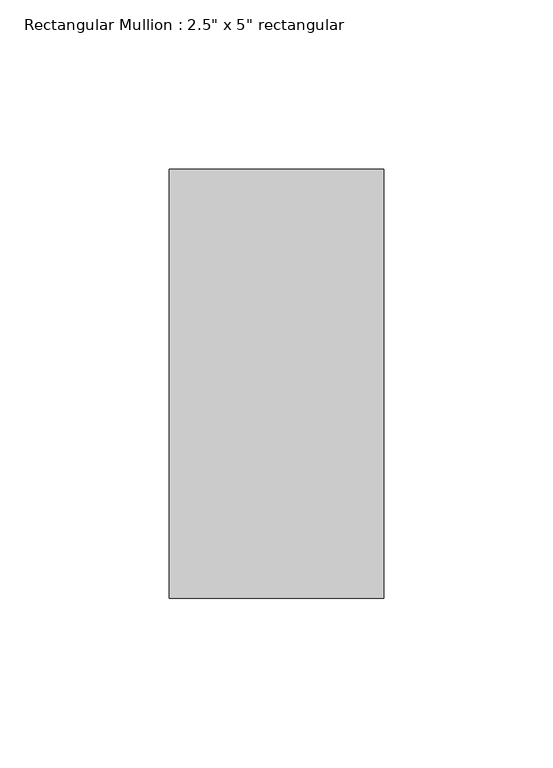
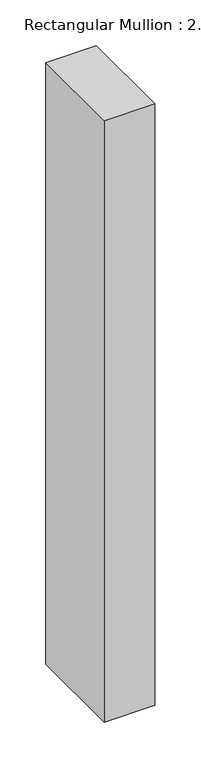
"""IFC4 building model written with IfcOpenShell, lengths in millimetres: member geometry."""

from ifc_helpers import new_model, si_unit, frame, origin, place, context, project, spatial, polyline, outline, extrude, source, transform, mapped, element, save


def member_b7f4e0be(model_context):
    return source(origin(), model_context, "Body", "SweptSolid", [
        extrude(outline(polyline([(0.0, 63.5), (0.0, -63.5), (-63.5, -63.5), (-63.5, 63.5), (0.0, 63.5)])), frame((0.0, 0.0, -799.240109), z_axis=(0.0, 0.0, 1.0), x_axis=(1.0, 0.0, 0.0)), (0.0, 0.0, 1.0), 799.240109),
    ])


if __name__ == "__main__":
    model = new_model("IFC4")
    model_context = context("Model", 3, world=origin())
    ifc_project = project(units=[si_unit("LENGTHUNIT", "METRE", prefix="MILLI")], contexts=[model_context])
    site = spatial("IfcSite", under=ifc_project)
    building = spatial("IfcBuilding", under=site)
    placement = place(None, origin())
    member_shape = member_b7f4e0be(model_context)
    element("IfcMember", 1, ObjectType="Rectangular Mullion : 2.5\" x 5\" rectangular", at=placement, inside=building, context=model_context, shape_type="MappedRepresentation", body=[
        mapped(member_shape, transform((0.0, 0.0, 0.0), x_axis=(1.0, 0.0, 0.0), y_axis=(0.0, 1.0, 0.0), z_axis=(0.0, 0.0, 1.0))),
    ])
    save(model, "model.ifc")

# Revit data of these elements
# Type "Rectangular Mullion : 2.5\" x 5\" rectangular"
#   built-in parameter 1007304 = 0.416667 (stored number, unit not read)
#   built-in parameter 1007301 = 0.104167 (stored number, unit not read)
#   built-in parameter 1007300 = 0.104167 (stored number, unit not read)
# Element 1 (IfcMember, "Rectangular Mullion : 2.5\" x 5\" rectangular")
#   Materials on its faces: "Aluminum"
# Materials
#   "Aluminum": class "Metal", colour RGB 247 247 247, transparency 0, Description = "Aluminum 6061", Cost = 0
